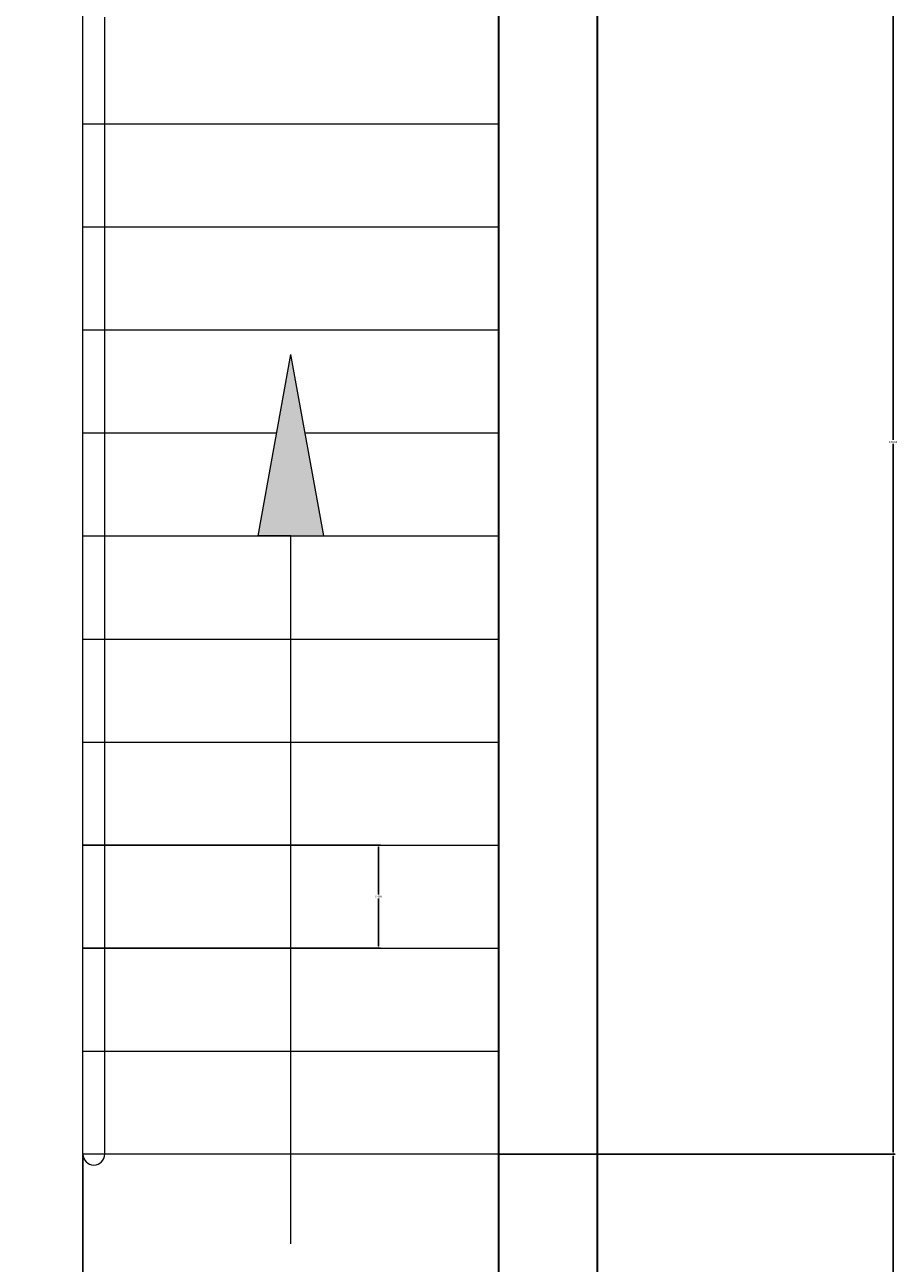
# Model space of a CAD drawing. Units: inches. Extents: x 2599 to 2953, y 557 to 1152.
# Tile 4 of 7: x 2874 to 2953, y 621 to 734. Entities that reach past the tile are written whole.
import ezdxf

# ---------------------------------------------------------------- set-up
doc = ezdxf.new("R2010")
doc.units = ezdxf.units.IN
for name, color, linetype, lineweight in [('A-ANNO-DIMS', 2, 'Continuous', 18), ('A-ANNO-SYMB', 7, 'Continuous', 18), ('A-FLOR-STRS', 254, 'Continuous', 18), ('A-WALL', 7, 'Continuous', 35)]:
    doc.layers.add(name, color=color, linetype=linetype, lineweight=lineweight)
doc.styles.get("Standard").update_dxf_attribs({"font": 'arial.ttf'})
doc.dimstyles.get("Standard").update_dxf_attribs({"dimtxt": 0.18, "dimasz": 0.18, "dimexe": 0.18, "dimexo": 0.0625, "dimgap": 0.09, "dimtad": 0, "dimtih": 1, "dimtoh": 1, "dimdec": 4, "dimzin": 0, "dimdsep": 46, "dimtxsty": 'Standard', "dimcen": 0.09, "dimadec": 0, "dimazin": 0, "dimtfac": 1, "dimtdec": 4, "dimtofl": 0, "dimtmove": 0, "dimatfit": 3, "dimfxl": 1, "dimtolj": 1, "dimtzin": 0, "dimarcsym": 0})

# ---------------------------------------------------------------- blocks, each defined once
blk = doc.blocks.new('*D21')
at = {"layer": 'A-ANNO-DIMS', "color": 0, "lineweight": -2, "transparency": 16777216}
for p, q in [((2625.92, 1124.28), (2625.92, 557.16)), ((2925.92, 584.28), (2925.92, 557.16)), ((2626.1, 557.34), (2775.63, 557.34)), ((2925.74, 557.34), (2776.21, 557.34))]:
    blk.add_line(p, q, dxfattribs=at)
at = {"layer": 'A-ANNO-DIMS', "color": 0, "transparency": 16777216}
for points in [[(2626.1, 557.37), (2626.1, 557.31), (2625.92, 557.34)], [(2925.74, 557.37), (2925.74, 557.31), (2925.92, 557.34)]]:
    blk.add_solid(points, dxfattribs=at)
at = {"layer": 'Defpoints', "color": 0, "transparency": 16777216}
for p in [(2625.92, 1124.34), (2925.92, 584.34), (2925.92, 557.34)]:
    blk.add_point(p, dxfattribs=at)
at = {"layer": 'A-ANNO-DIMS', "color": 0, "transparency": 16777216, "insert": (2775.92, 557.34), "char_height": 0.18, "attachment_point": 5}
blk.add_mtext('\\A1;300', dxfattribs=at)
blk = doc.blocks.new('*D40')
at = {"layer": 'A-ANNO-DIMS', "color": 0, "lineweight": -2, "transparency": 16777216}
for p, q in [((2878.92, 631.2), (2878.92, 604.08)), ((2916.92, 631.2), (2916.92, 604.08)), ((2879.1, 604.26), (2897.7, 604.26)), ((2916.74, 604.26), (2898.14, 604.26))]:
    blk.add_line(p, q, dxfattribs=at)
at = {"layer": 'A-ANNO-DIMS', "color": 0, "transparency": 16777216}
for points in [[(2879.1, 604.29), (2879.1, 604.23), (2878.92, 604.26)], [(2916.74, 604.29), (2916.74, 604.23), (2916.92, 604.26)]]:
    blk.add_solid(points, dxfattribs=at)
at = {"layer": 'Defpoints', "color": 0, "transparency": 16777216}
for p in [(2878.92, 631.26), (2916.92, 631.26), (2878.92, 604.26)]:
    blk.add_point(p, dxfattribs=at)
at = {"layer": 'A-ANNO-DIMS', "color": 0, "transparency": 16777216, "insert": (2897.92, 604.26), "char_height": 0.18, "attachment_point": 5}
blk.add_mtext('\\A1;38', dxfattribs=at)
blk = doc.blocks.new('*D41')
at = {"layer": 'A-ANNO-DIMS', "color": 0, "lineweight": -2, "transparency": 16777216}
for p, q in [((2916.98, 761.34), (2953.1, 761.34)), ((2952.92, 761.16), (2952.92, 696.48)), ((2952.92, 631.44), (2952.92, 696.12)), ((2916.98, 631.26), (2953.1, 631.26))]:
    blk.add_line(p, q, dxfattribs=at)
at = {"layer": 'A-ANNO-DIMS', "color": 0, "transparency": 16777216}
for points in [[(2952.89, 761.16), (2952.95, 761.16), (2952.92, 761.34)], [(2952.89, 631.44), (2952.95, 631.44), (2952.92, 631.26)]]:
    blk.add_solid(points, dxfattribs=at)
at = {"layer": 'Defpoints', "color": 0, "transparency": 16777216}
for p in [(2916.92, 761.34), (2952.92, 761.34), (2916.92, 631.26)]:
    blk.add_point(p, dxfattribs=at)
at = {"layer": 'A-ANNO-DIMS', "color": 0, "transparency": 16777216, "insert": (2952.92, 696.3), "char_height": 0.18, "attachment_point": 5}
blk.add_mtext('\\A1;130.08', dxfattribs=at)
blk = doc.blocks.new('*D42')
at = {"layer": 'A-ANNO-DIMS', "color": 0, "lineweight": -2, "transparency": 16777216}
for p, q in [((2916.98, 631.26), (2953.1, 631.26)), ((2952.92, 631.08), (2952.92, 607.98)), ((2952.92, 584.52), (2952.92, 607.62)), ((2916.98, 584.34), (2953.1, 584.34))]:
    blk.add_line(p, q, dxfattribs=at)
at = {"layer": 'A-ANNO-DIMS', "color": 0, "transparency": 16777216}
for points in [[(2952.89, 631.08), (2952.95, 631.08), (2952.92, 631.26)], [(2952.89, 584.52), (2952.95, 584.52), (2952.92, 584.34)]]:
    blk.add_solid(points, dxfattribs=at)
at = {"layer": 'Defpoints', "color": 0, "transparency": 16777216}
for p in [(2916.92, 631.26), (2952.92, 631.26), (2916.92, 584.34)]:
    blk.add_point(p, dxfattribs=at)
at = {"layer": 'A-ANNO-DIMS', "color": 0, "transparency": 16777216, "insert": (2952.92, 607.8), "char_height": 0.18, "attachment_point": 5}
blk.add_mtext('\\A1;46.92', dxfattribs=at)
blk = doc.blocks.new('*D43')
at = {"layer": 'A-ANNO-DIMS', "color": 0, "lineweight": -2, "transparency": 16777216}
for p, q in [((2878.98, 659.49), (2906.1, 659.49)), ((2905.92, 659.31), (2905.92, 654.97)), ((2905.92, 650.26), (2905.92, 654.6)), ((2878.98, 650.08), (2906.1, 650.08))]:
    blk.add_line(p, q, dxfattribs=at)
at = {"layer": 'A-ANNO-DIMS', "color": 0, "transparency": 16777216}
for points in [[(2905.89, 659.31), (2905.95, 659.31), (2905.92, 659.49)], [(2905.89, 650.26), (2905.95, 650.26), (2905.92, 650.08)]]:
    blk.add_solid(points, dxfattribs=at)
at = {"layer": 'Defpoints', "color": 0, "transparency": 16777216}
for p in [(2878.92, 659.49), (2878.92, 650.08), (2905.92, 650.08)]:
    blk.add_point(p, dxfattribs=at)
at = {"layer": 'A-ANNO-DIMS', "color": 0, "transparency": 16777216, "insert": (2905.92, 654.78), "char_height": 0.18, "attachment_point": 5}
blk.add_mtext('\\A1;9.408', dxfattribs=at)

msp = doc.modelspace()

# ---------------------------------------------------------------- hatches: boundary and pattern name
at = {"layer": 'A-ANNO-SYMB'}
h = msp.add_hatch(color=256, dxfattribs=at)
h.dxf.hatch_style = 1
h.paths.add_polyline_path([(2897.9211, 704.3002), (2894.9211, 687.7121), (2897.9211, 687.7121), (2900.9211, 687.7121)])

# ---------------------------------------------------------------- linework, layer by layer
for p, q in [((2894.9211, 687.7121), (2897.9211, 704.3002)), ((2900.9211, 687.7121), (2897.9211, 704.3002)), ((2897.9211, 687.7121), (2894.9211, 687.7121)), ((2897.9211, 623.0684), (2897.9211, 687.7121)), ((2897.9211, 687.7121), (2900.9211, 687.7121))]:
    msp.add_line(p, q, dxfattribs=at)
at = {"layer": 'A-FLOR-STRS'}
for p, q in [((2878.9211, 631.2641), (2878.9211, 761.3417)), ((2880.9211, 631.2641), (2880.9211, 735.0939)), ((2878.9211, 725.3441), (2916.9211, 725.3441)), ((2878.9211, 715.9361), (2916.9211, 715.9361)), ((2878.9211, 706.5281), (2916.9211, 706.5281)), ((2878.9211, 697.1201), (2896.6226, 697.1201)), ((2899.2196, 697.1201), (2916.9211, 697.1201)), ((2878.9211, 687.7121), (2916.9211, 687.7121)), ((2878.9211, 678.3041), (2916.9211, 678.3041)), ((2878.9211, 668.8961), (2916.9211, 668.8961)), ((2878.9211, 659.4881), (2916.9211, 659.4881)), ((2878.9211, 650.0801), (2916.9211, 650.0801)), ((2878.9211, 640.6721), (2916.9211, 640.6721)), ((2880.9211, 631.2641), (2878.9211, 631.2641)), ((2916.9211, 631.2641), (2880.9211, 631.2641))]:
    msp.add_line(p, q, dxfattribs=at)
msp.add_arc((2879.9211, 631.2641), 1, 180, 0, dxfattribs=at)
at = {"layer": 'A-WALL'}
for p, q in [((2925.9211, 584.3417), (2925.9211, 1124.3417)), ((2916.9211, 610.5917), (2916.9211, 761.3417))]:
    msp.add_line(p, q, dxfattribs=at)

# ---------------------------------------------------------------- dimensions: what is measured, and where the dimension line sits
at = {"layer": 'A-ANNO-DIMS'}
dim = msp.add_linear_dim(base=(2925.9211, 557.3382), p1=(2625.9211, 1124.3417), p2=(2925.9211, 584.3417), dimstyle='Standard', override={"dimdec": 0, "dimlfac": 1, "dimrnd": 0, "dimzin": 0, "dimdsep": 46, "dimlunit": 2}, dxfattribs=at)
dim.commit()
dim.dimension.update_dxf_attribs({"geometry": '*D21', "text_midpoint": (2775.9211, 557.3382)})
for base, p1, p2, angle, override, picture, middle in [((2952.9246, 761.3417), (2916.9211, 631.2641), (2916.9211, 761.3417), 90, {"dimdec": 2, "dimlfac": 1, "dimrnd": 0, "dimzin": 0, "dimdsep": 46, "dimlunit": 2}, '*D41', (2952.9246, 696.3029)), ((2905.9246, 650.0801), (2878.9211, 659.4881), (2878.9211, 650.0801), 270, {"dimdec": 3, "dimlfac": 1, "dimrnd": 0, "dimzin": 0, "dimdsep": 46, "dimlunit": 2}, '*D43', (2905.9246, 654.7841)), ((2878.9211, 604.2606), (2916.9211, 631.2641), (2878.9211, 631.2641), 180, {"dimdec": 0, "dimlfac": 1, "dimrnd": 0, "dimzin": 0, "dimdsep": 46, "dimlunit": 2}, '*D40', (2897.9211, 604.2606)), ((2952.9246, 631.2641), (2916.9211, 584.3417), (2916.9211, 631.2641), 90, {"dimdec": 2, "dimlfac": 1, "dimrnd": 0, "dimzin": 0, "dimdsep": 46, "dimlunit": 2}, '*D42', (2952.9246, 607.8029))]:
    dim = msp.add_linear_dim(base=base, p1=p1, p2=p2, angle=angle, dimstyle='Standard', override=override, dxfattribs=at)
    dim.commit()
    dim.dimension.update_dxf_attribs({"geometry": picture, "text_midpoint": middle})

doc.saveas('drawing.dxf')
